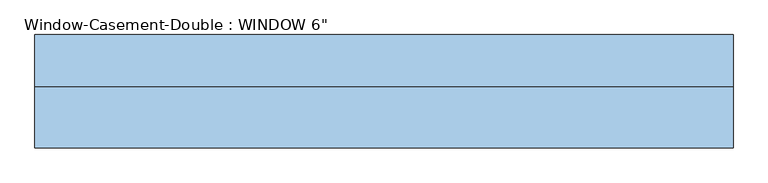
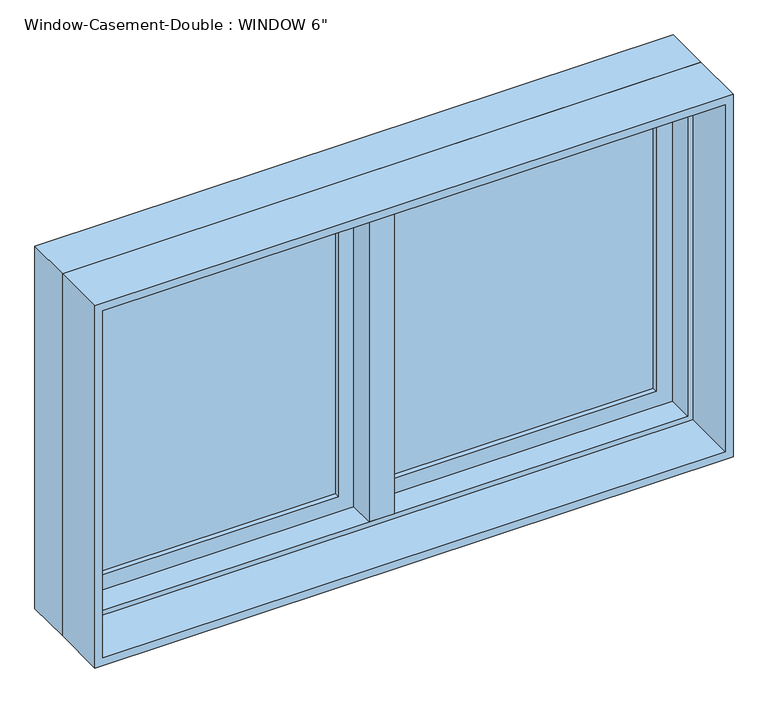
"""IFC4 building model written with IfcOpenShell, lengths in millimetres: window geometry."""

from ifc_helpers import new_model, si_unit, frame, origin, place, context, project, spatial, polyline, outline, extrude, faceted_brep, source, transform, mapped, element, save


def window_c1d95f0f(model_context):
    return source(origin(), model_context, "Body", "SolidModel", [
        faceted_brep([(9.525, 133.35, 1816.1), (-9.525, 133.35, 1816.1), (-9.525, 82.55, 1816.1), (9.525, 82.55, 1816.1), (9.525, 133.35, 927.1), (9.525, 82.55, 927.1), (-9.525, 82.55, 927.1), (-9.525, 133.35, 927.1), (-9.525, 82.55, 946.15), (-9.525, 82.55, 1797.05), (-30.1625, 82.55, 946.15), (-30.1625, 82.55, 1797.05), (-30.1625, 19.05, 946.15), (-30.1625, 19.05, 1797.05), (30.1625, 19.05, 946.15), (30.1625, 19.05, 1797.05), (30.1625, 82.55, 946.15), (30.1625, 82.55, 1797.05), (9.525, 82.55, 946.15), (9.525, 82.55, 1797.05)], [[[0, 1, 2, 3]], [[4, 5, 6, 7]], [[1, 0, 4, 7]], [[2, 1, 7, 6, 8, 9]], [[9, 8, 10, 11]], [[11, 10, 12, 13]], [[13, 12, 14, 15]], [[15, 14, 16, 17]], [[17, 16, 18, 19]], [[0, 3, 19, 18, 5, 4]], [[18, 8, 6, 5]], [[9, 19, 3, 2]], [[8, 18, 16, 14, 12, 10]], [[19, 9, 11, 13, 15, 17]]]),
        extrude(outline(polyline([(-66.675, 114.3), (-66.675, 107.95), (-692.15, 107.95), (-692.15, 114.3), (-66.675, 114.3)])), frame((0.0, 0.0, 984.25), z_axis=(0.0, 0.0, 1.0), x_axis=(1.0, 0.0, 0.0)), (0.0, 0.0, 1.0), 774.7),
        extrude(outline(polyline([(-692.15, 95.25), (-692.15, 101.6), (-66.675, 101.6), (-66.675, 95.25), (-692.15, 95.25)])), frame((0.0, 0.0, 984.25), z_axis=(0.0, 0.0, 1.0), x_axis=(1.0, 0.0, 0.0)), (0.0, 0.0, 1.0), 774.7),
        extrude(outline(polyline([(692.15, 114.3), (692.15, 107.95), (66.675, 107.95), (66.675, 114.3), (692.15, 114.3)])), frame((0.0, 0.0, 984.25), z_axis=(0.0, 0.0, 1.0), x_axis=(1.0, 0.0, 0.0)), (0.0, 0.0, 1.0), 774.7),
        extrude(outline(polyline([(66.675, 95.25), (66.675, 101.6), (692.15, 101.6), (692.15, 95.25), (66.675, 95.25)])), frame((0.0, 0.0, 984.25), z_axis=(0.0, 0.0, 1.0), x_axis=(1.0, 0.0, 0.0)), (0.0, 0.0, 1.0), 774.7),
        extrude(outline(polyline([(1816.1, -749.3), (927.1, -749.3), (927.1, -9.525), (1816.1, -9.525), (1816.1, -749.3)]), holes=[polyline([(1758.95, -66.675), (984.25, -66.675), (984.25, -692.15), (1758.95, -692.15), (1758.95, -66.675)])]), frame((0.0, 82.55, 0.0), z_axis=(0.0, 1.0, 0.0), x_axis=(0.0, 0.0, 1.0)), (0.0, 0.0, 1.0), 44.45),
        extrude(outline(polyline([(927.1, 749.3), (1816.1, 749.3), (1816.1, 9.525), (927.1, 9.525), (927.1, 749.3)]), holes=[polyline([(984.25, 66.675), (1758.95, 66.675), (1758.95, 692.15), (984.25, 692.15), (984.25, 66.675)])]), frame((0.0, 82.55, 0.0), z_axis=(0.0, 1.0, 0.0), x_axis=(0.0, 0.0, 1.0)), (0.0, 0.0, 1.0), 44.45),
        extrude(outline(polyline([(1828.8, -762.0), (914.4, -762.0), (914.4, 762.0), (1828.8, 762.0), (1828.8, -762.0)]), holes=[polyline([(1809.75, 742.95), (933.45, 742.95), (933.45, -742.95), (1809.75, -742.95), (1809.75, 742.95)])]), frame((0.0, -114.3, 0.0), z_axis=(0.0, 1.0, 0.0), x_axis=(0.0, 0.0, 1.0)), (0.0, 0.0, 1.0), 133.35),
        faceted_brep([(730.25, 82.55, 1797.05), (730.25, 19.05, 1797.05), (-730.25, 19.05, 1797.05), (-730.25, 82.55, 1797.05), (749.3, 133.35, 1816.1), (749.3, 82.55, 1816.1), (-749.3, 82.55, 1816.1), (-749.3, 133.35, 1816.1), (762.0, 19.05, 1828.8), (762.0, 133.35, 1828.8), (-762.0, 133.35, 1828.8), (-762.0, 19.05, 1828.8), (-730.25, 19.05, 946.15), (-730.25, 82.55, 946.15), (-749.3, 82.55, 927.1), (-749.3, 133.35, 927.1), (-762.0, 133.35, 914.4), (-762.0, 19.05, 914.4), (730.25, 19.05, 946.15), (730.25, 82.55, 946.15), (749.3, 82.55, 927.1), (749.3, 133.35, 927.1), (762.0, 133.35, 914.4), (762.0, 19.05, 914.4)], [[[0, 1, 2, 3]], [[4, 5, 6, 7]], [[8, 9, 10, 11]], [[3, 2, 12, 13]], [[7, 6, 14, 15]], [[11, 10, 16, 17]], [[13, 12, 18, 19]], [[15, 14, 20, 21]], [[17, 16, 22, 23]], [[11, 17, 23, 8], [1, 18, 12, 2]], [[19, 18, 1, 0]], [[5, 20, 14, 6], [3, 13, 19, 0]], [[21, 20, 5, 4]], [[23, 22, 9, 8]], [[9, 22, 16, 10], [7, 15, 21, 4]]]),
    ])


if __name__ == "__main__":
    model = new_model("IFC4")
    model_context = context("Model", 3, world=origin())
    ifc_project = project(units=[si_unit("LENGTHUNIT", "METRE", prefix="MILLI")], contexts=[model_context])
    site = spatial("IfcSite", under=ifc_project)
    building = spatial("IfcBuilding", under=site)
    placement = place(None, origin())
    window_shape = window_c1d95f0f(model_context)
    element("IfcWindow", 1, ObjectType="Window-Casement-Double : WINDOW 6\"", at=placement, inside=building, context=model_context, shape_type="MappedRepresentation", body=[
        mapped(window_shape, transform((0.0, 0.0, 0.0), x_axis=(1.0, 0.0, 0.0), y_axis=(0.0, 1.0, 0.0), z_axis=(0.0, 0.0, 1.0))),
    ])
    save(model, "model.ifc")

# Revit data of these elements
# Type "Window-Casement-Double : WINDOW 6\""
#   Type Mark = "18"
#   Fire Rating = "0.5h"
#   Assembly Code = "B2020100"
#   Analytic Construction = "Double glazing - domestic"
#   Frame Extension [instance default] = 0' - 0 1/4"
#   Window Inset [instance default] = 0' - 0"
#   Wall Thickness [instance default] = 0' - 6"
#   Interior Wall Closure [instance default] = 0' - 2 1/4"
#   Half Width = 2' - 6"
#   Visual Light Transmittance = 0.81
#   Thermal Resistance (R) = 1.8146 (h·ft²·°F)/BTU
#   Solar Heat Gain Coefficient = 0.76
#   Rough Width = 5' - 0 1/2"
#   Rough Height = 3' - 0 1/2"
#   Height = 3' - 0"
#   Heat Transfer Coefficient (U) = 0.5511 BTU/(h·ft²·°F)
#   Exterior Wall Closure [instance default] = 0' - 1 1/4"
#   Extension Jamb [instance default] = 0' - 2 1/4"
#   Default Sill Height = 3' - 0"
#   Width = 5' - 0"
#   Muntin Visibility = yes
#   Interior Trim Visibility [instance default] = yes
#   Exterior Trim Visibility [instance default] = yes
#   Extension Jamb Visibility [instance default] = yes
#   Interior Trim Material = Wood - Stained
#   Muntin Pattern = Muntin Pattern_2x2 : Muntin Pattern_2x2
#   Interior Trim = Trim-Window-Interior-Flat : Picture Frame
#   Interior Frame Material = Wood - Stained
#   Glass Panel Material = Glass
#   Exterior Trim Material = Clad - White
#   Exterior Trim = Trim-Window-Exterior-Flat : with Sill
#   Exterior Frame Material = Clad - White
#   Wall Closure = (empty or 0)
# Element 1 (IfcWindow, "Window-Casement-Double : WINDOW 6\"")
#   Wall Thickness = 0' - 9"
#   Extension Jamb = 0' - 5 1/4"
#   Materials on its faces: "Wood - Stained", "Glass", "Clad - White"
# Materials
#   "Wood - Stained": class "Wood", colour RGB 224 178 126, transparency 0, Cost = 0
#   "Glass": class "Glass", colour RGB 0 128 192, transparency 0.75, Description = "Soda Lime Glass", Cost = 0
#   "Clad - White": class "Wood", colour RGB 242 242 238, transparency 0, Cost = 0
